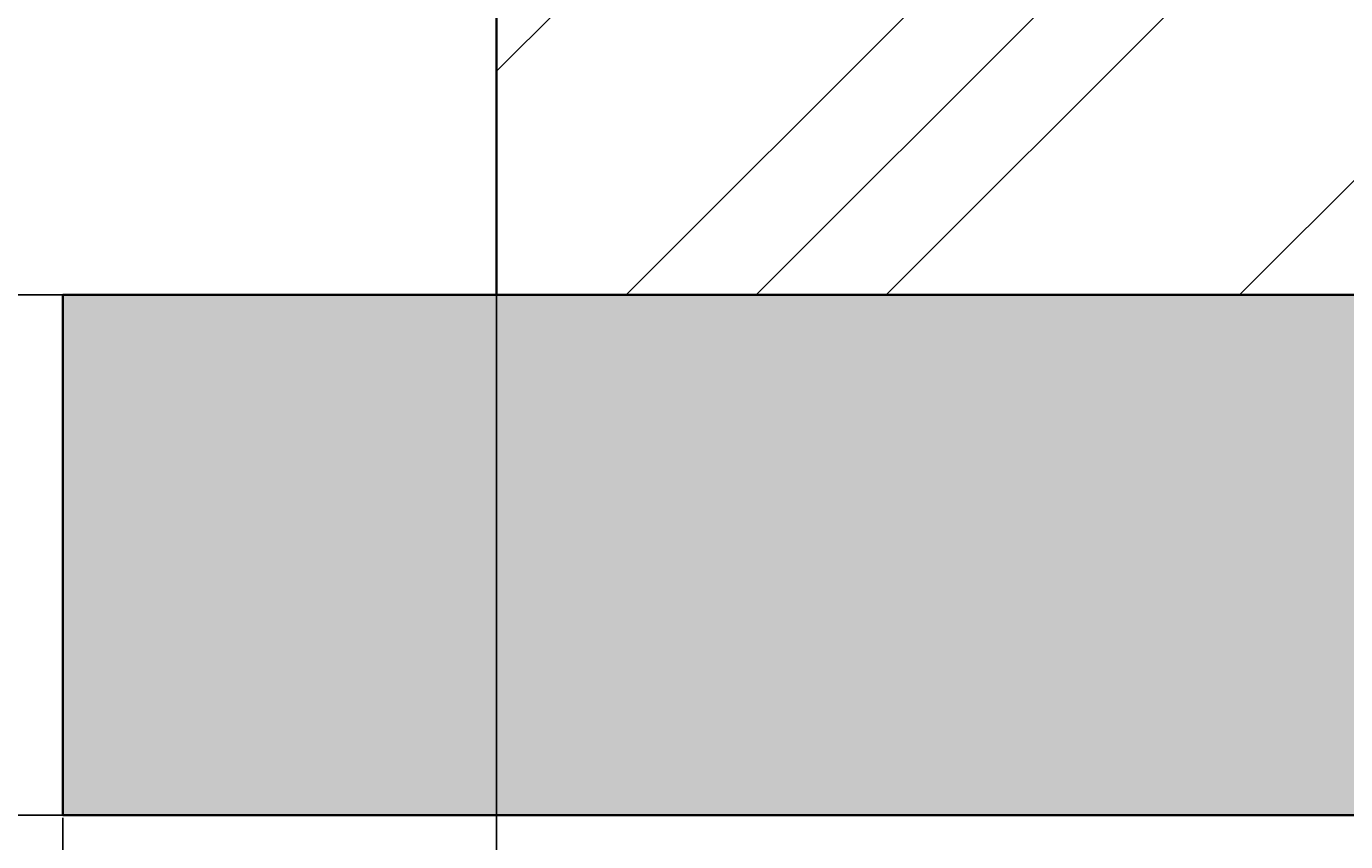
# Model space of a CAD drawing. Units: inches. Extents: x -128 to 854, y -395 to 398.
# Tile 4 of 61: x -77 to -47, y -359 to -340. Entities that reach past the tile are written whole.
import ezdxf

# ---------------------------------------------------------------- set-up
doc = ezdxf.new("R2010")
doc.units = ezdxf.units.IN
doc.header["$MEASUREMENT"] = 0
for name, color, linetype, lineweight in [('A-ANNO-DIMS', 2, 'Continuous', 18), ('A-SECT-PATT', 8, 'Continuous', 13), ('S-FNDN', 2, 'Continuous', 35), ('S-FNDN-PATT', 8, 'Continuous', 13)]:
    doc.layers.add(name, color=color, linetype=linetype, lineweight=lineweight)
doc.styles.get("Standard").update_dxf_attribs({"font": 'arial.ttf'})
doc.dimstyles.get("Standard").update_dxf_attribs({"dimtxt": 0.18, "dimasz": 0.18, "dimexe": 0.18, "dimexo": 0.0625, "dimgap": 0.09, "dimtad": 0, "dimtih": 1, "dimtoh": 1, "dimdec": 1, "dimzin": 0, "dimdsep": 46, "dimlunit": 4, "dimtxsty": 'Standard', "dimcen": 0.09, "dimclrd": 1, "dimclre": 2, "dimclrt": 6, "dimadec": 0, "dimazin": 0, "dimtfac": 1, "dimtdec": 1, "dimtofl": 0, "dimtmove": 0, "dimatfit": 3, "dimfxl": 1, "dimtfill": 2, "dimtfillclr": 3, "dimtolj": 1, "dimtzin": 0, "dimarcsym": 0})

# ---------------------------------------------------------------- blocks, each defined once
blk = doc.blocks.new('*D121')
at = {"layer": 'A-ANNO-DIMS', "color": 2, "lineweight": -2, "transparency": 16777216}
for p, q in [((-56.223, -298.019), (-128.041, -298.019)), ((-76.223, -358.019), (-128.041, -358.019))]:
    blk.add_line(p, q, dxfattribs=at)
at = {"layer": 'A-ANNO-DIMS', "color": 1, "lineweight": -2, "transparency": 16777216}
for p, q in [((-127.861, -298.199), (-127.861, -327.837)), ((-127.861, -357.839), (-127.861, -328.201))]:
    blk.add_line(p, q, dxfattribs=at)
at = {"layer": 'A-ANNO-DIMS', "color": 1, "transparency": 16777216}
for points in [[(-127.891, -298.199), (-127.831, -298.199), (-127.861, -298.019)], [(-127.891, -357.839), (-127.831, -357.839), (-127.861, -358.019)]]:
    blk.add_solid(points, dxfattribs=at)
at = {"layer": 'Defpoints', "color": 0, "transparency": 16777216}
for p in [(-56.161, -298.019), (-127.861, -358.019), (-76.161, -358.019)]:
    blk.add_point(p, dxfattribs=at)
at = {"layer": 'A-ANNO-DIMS', "color": 6, "transparency": 16777216, "insert": (-127.861, -328.019), "char_height": 0.18, "attachment_point": 5, "bg_fill": 1, "box_fill_scale": 1.25, "bg_fill_color": 3, "bg_fill_transparency": 0}
blk.add_mtext('\\A1;5\'-0"', dxfattribs=at)
blk = doc.blocks.new('*D122')
at = {"layer": 'A-ANNO-DIMS', "color": 2, "lineweight": -2, "transparency": 16777216}
for p, q in [((-76.161, -358.082), (-76.161, -381.899)), ((-17.161, -358.082), (-17.161, -381.899))]:
    blk.add_line(p, q, dxfattribs=at)
at = {"layer": 'A-ANNO-DIMS', "color": 1, "lineweight": -2, "transparency": 16777216}
for p, q in [((-75.981, -381.719), (-47.064, -381.719)), ((-17.341, -381.719), (-46.258, -381.719))]:
    blk.add_line(p, q, dxfattribs=at)
at = {"layer": 'A-ANNO-DIMS', "color": 1, "transparency": 16777216}
for points in [[(-75.981, -381.689), (-75.981, -381.749), (-76.161, -381.719)], [(-17.341, -381.689), (-17.341, -381.749), (-17.161, -381.719)]]:
    blk.add_solid(points, dxfattribs=at)
at = {"layer": 'Defpoints', "color": 0, "transparency": 16777216}
for p in [(-76.161, -358.019), (-17.161, -358.019), (-17.161, -381.719)]:
    blk.add_point(p, dxfattribs=at)
at = {"layer": 'A-ANNO-DIMS', "color": 6, "transparency": 16777216, "insert": (-46.661, -381.719), "char_height": 0.18, "attachment_point": 5, "bg_fill": 1, "box_fill_scale": 1.25, "bg_fill_color": 3, "bg_fill_transparency": 0}
blk.add_mtext('\\A1;4\'-11"', dxfattribs=at)
blk = doc.blocks.new('*D128')
at = {"layer": 'A-ANNO-DIMS', "color": 2, "lineweight": -2, "transparency": 16777216}
for p, q in [((-17.223, -346.019), (-128.041, -346.019)), ((-17.223, -358.019), (-128.041, -358.019))]:
    blk.add_line(p, q, dxfattribs=at)
at = {"layer": 'A-ANNO-DIMS', "color": 1, "lineweight": -2, "transparency": 16777216}
for p, q in [((-127.861, -346.199), (-127.861, -351.837)), ((-127.861, -357.839), (-127.861, -352.201))]:
    blk.add_line(p, q, dxfattribs=at)
at = {"layer": 'A-ANNO-DIMS', "color": 1, "transparency": 16777216}
for points in [[(-127.891, -346.199), (-127.831, -346.199), (-127.861, -346.019)], [(-127.891, -357.839), (-127.831, -357.839), (-127.861, -358.019)]]:
    blk.add_solid(points, dxfattribs=at)
at = {"layer": 'Defpoints', "color": 0, "transparency": 16777216}
for p in [(-127.861, -346.019), (-17.161, -346.019), (-17.161, -358.019)]:
    blk.add_point(p, dxfattribs=at)
at = {"layer": 'A-ANNO-DIMS', "color": 6, "transparency": 16777216, "insert": (-127.861, -352.019), "char_height": 0.18, "attachment_point": 5, "bg_fill": 1, "box_fill_scale": 1.25, "bg_fill_color": 3, "bg_fill_transparency": 0}
blk.add_mtext('\\A1;1\'-0"', dxfattribs=at)
blk = doc.blocks.new('*D129')
at = {"layer": 'A-ANNO-DIMS', "color": 2, "lineweight": -2, "transparency": 16777216}
for p, q in [((-27.223, -322.019), (-128.041, -322.019)), ((-27.223, -346.019), (-128.041, -346.019))]:
    blk.add_line(p, q, dxfattribs=at)
at = {"layer": 'A-ANNO-DIMS', "color": 1, "lineweight": -2, "transparency": 16777216}
for p, q in [((-127.861, -322.199), (-127.861, -333.837)), ((-127.861, -345.839), (-127.861, -334.201))]:
    blk.add_line(p, q, dxfattribs=at)
at = {"layer": 'A-ANNO-DIMS', "color": 1, "transparency": 16777216}
for points in [[(-127.891, -322.199), (-127.831, -322.199), (-127.861, -322.019)], [(-127.891, -345.839), (-127.831, -345.839), (-127.861, -346.019)]]:
    blk.add_solid(points, dxfattribs=at)
at = {"layer": 'Defpoints', "color": 0, "transparency": 16777216}
for p in [(-127.861, -322.019), (-27.161, -322.019), (-27.161, -346.019)]:
    blk.add_point(p, dxfattribs=at)
at = {"layer": 'A-ANNO-DIMS', "color": 6, "transparency": 16777216, "insert": (-127.861, -334.019), "char_height": 0.18, "attachment_point": 5, "bg_fill": 1, "box_fill_scale": 1.25, "bg_fill_color": 3, "bg_fill_transparency": 0}
blk.add_mtext('\\A1;2\'-0"', dxfattribs=at)
blk = doc.blocks.new('*D130')
at = {"layer": 'A-ANNO-DIMS', "color": 2, "lineweight": -2, "transparency": 16777216}
for p, q in [((-66.161, -322.082), (-66.161, -381.899)), ((-27.161, -322.082), (-27.161, -381.899))]:
    blk.add_line(p, q, dxfattribs=at)
at = {"layer": 'A-ANNO-DIMS', "color": 1, "lineweight": -2, "transparency": 16777216}
for p, q in [((-65.981, -381.719), (-46.99, -381.719)), ((-27.341, -381.719), (-46.332, -381.719))]:
    blk.add_line(p, q, dxfattribs=at)
at = {"layer": 'A-ANNO-DIMS', "color": 1, "transparency": 16777216}
for points in [[(-65.981, -381.689), (-65.981, -381.749), (-66.161, -381.719)], [(-27.341, -381.689), (-27.341, -381.749), (-27.161, -381.719)]]:
    blk.add_solid(points, dxfattribs=at)
at = {"layer": 'Defpoints', "color": 0, "transparency": 16777216}
for p in [(-66.161, -322.019), (-27.161, -322.019), (-27.161, -381.719)]:
    blk.add_point(p, dxfattribs=at)
at = {"layer": 'A-ANNO-DIMS', "color": 6, "transparency": 16777216, "insert": (-46.661, -381.719), "char_height": 0.18, "attachment_point": 5, "bg_fill": 1, "box_fill_scale": 1.25, "bg_fill_color": 3, "bg_fill_transparency": 0}
blk.add_mtext('\\A1;3\'-3"', dxfattribs=at)

msp = doc.modelspace()

# ---------------------------------------------------------------- hatches: boundary and pattern name
at = {"layer": 'A-SECT-PATT'}
h = msp.add_hatch(dxfattribs=at)
h.set_pattern_fill('GOST_GROUND', color=256)
h.set_pattern_definition([(45, (0, 0), (14.14214, -9e-16), [20]), (45, (3, 0), (14.14214, -9e-16), [20]), (45, (6, 0), (14.14214, -9e-16), [20])])
h.paths.add_polyline_path([(-27.161, -322.019), (-37.161, -322.019), (-37.161, -298.019), (-56.161, -298.019), (-56.161, -322.019), (-66.161, -322.019), (-66.161, -346.019), (-27.161, -346.019)])
h.paths.add_polyline_path([(170.839, -322.019), (160.839, -322.019), (160.839, -298.019), (155.839, -298.019), (141.839, -298.019), (141.839, -322.019), (131.839, -322.019), (131.839, -346.019), (170.839, -346.019)])
h.paths.add_polyline_path([(327.839, -322.019), (317.839, -322.019), (317.839, -298.019), (312.839, -298.019), (298.839, -298.019), (298.839, -322.019), (288.839, -322.019), (288.839, -346.019), (327.839, -346.019)])
h.paths.add_polyline_path([(-37.161, -274.019), (-56.161, -274.019), (-56.161, -298.019), (-37.161, -298.019)])
h.paths.add_polyline_path([(-37.161, -207.019), (-56.161, -207.019), (-56.161, -226.019), (-37.161, -226.019)])
h.paths.add_polyline_path([(160.839, -274.019), (141.839, -274.019), (141.839, -298.019), (155.839, -298.019), (160.839, -298.019)])
at = {"layer": 'S-FNDN-PATT'}
h = msp.add_hatch(dxfattribs=at)
h.set_pattern_fill('AR-CONC', color=256)
h.paths.add_polyline_path([(-17.161, -346.019), (-27.161, -346.019), (-66.161, -346.019), (-76.161, -346.019), (-76.161, -358.019), (-17.161, -358.019)])
h.paths.add_polyline_path([(180.839, -346.019), (170.839, -346.019), (131.839, -346.019), (121.839, -346.019), (121.839, -358.019), (180.839, -358.019)])
h.paths.add_polyline_path([(337.839, -346.019), (327.839, -346.019), (288.839, -346.019), (278.839, -346.019), (278.839, -358.019), (337.839, -358.019)])

# ---------------------------------------------------------------- linework, layer by layer
at = {"layer": 'S-FNDN'}
for p, q in [((-66.161, -322.019), (-66.161, -346.019)), ((-66.161, -346.019), (-76.161, -346.019)), ((-76.161, -346.019), (-76.161, -358.019)), ((-66.161, -346.019), (-27.161, -346.019)), ((-76.161, -358.019), (-17.161, -358.019))]:
    msp.add_line(p, q, dxfattribs=at)

# ---------------------------------------------------------------- dimensions: what is measured, and where the dimension line sits
at = {"layer": 'A-ANNO-DIMS'}
for base, p1, p2, picture, middle in [((-127.861, -358.019), (-56.161, -298.019), (-76.161, -358.019), '*D121', (-127.861, -328.019)), ((-127.861, -322.019), (-27.161, -346.019), (-27.161, -322.019), '*D129', (-127.861, -334.019)), ((-127.861, -346.019), (-17.161, -358.019), (-17.161, -346.019), '*D128', (-127.861, -352.019))]:
    dim = msp.add_linear_dim(base=base, p1=p1, p2=p2, angle=90, dimstyle='Standard', override={"dimdec": 1, "dimlfac": 1, "dimrnd": 0, "dimzin": 1, "dimdsep": 46, "dimlunit": 4, "dimfrac": 2}, dxfattribs=at)
    dim.commit()
    dim.dimension.update_dxf_attribs({"geometry": picture, "text_midpoint": middle})
for base, p1, p2, picture in [((-27.161, -381.719), (-66.161, -322.019), (-27.161, -322.019), '*D130'), ((-17.161, -381.719), (-76.161, -358.019), (-17.161, -358.019), '*D122')]:
    dim = msp.add_linear_dim(base=base, p1=p1, p2=p2, dimstyle='Standard', override={"dimdec": 1, "dimlfac": 1, "dimrnd": 0, "dimzin": 1, "dimdsep": 46, "dimlunit": 4, "dimfrac": 2}, dxfattribs=at)
    dim.commit()
    dim.dimension.update_dxf_attribs({"geometry": picture, "text_midpoint": (-46.661, -381.719)})

doc.saveas('drawing.dxf')
